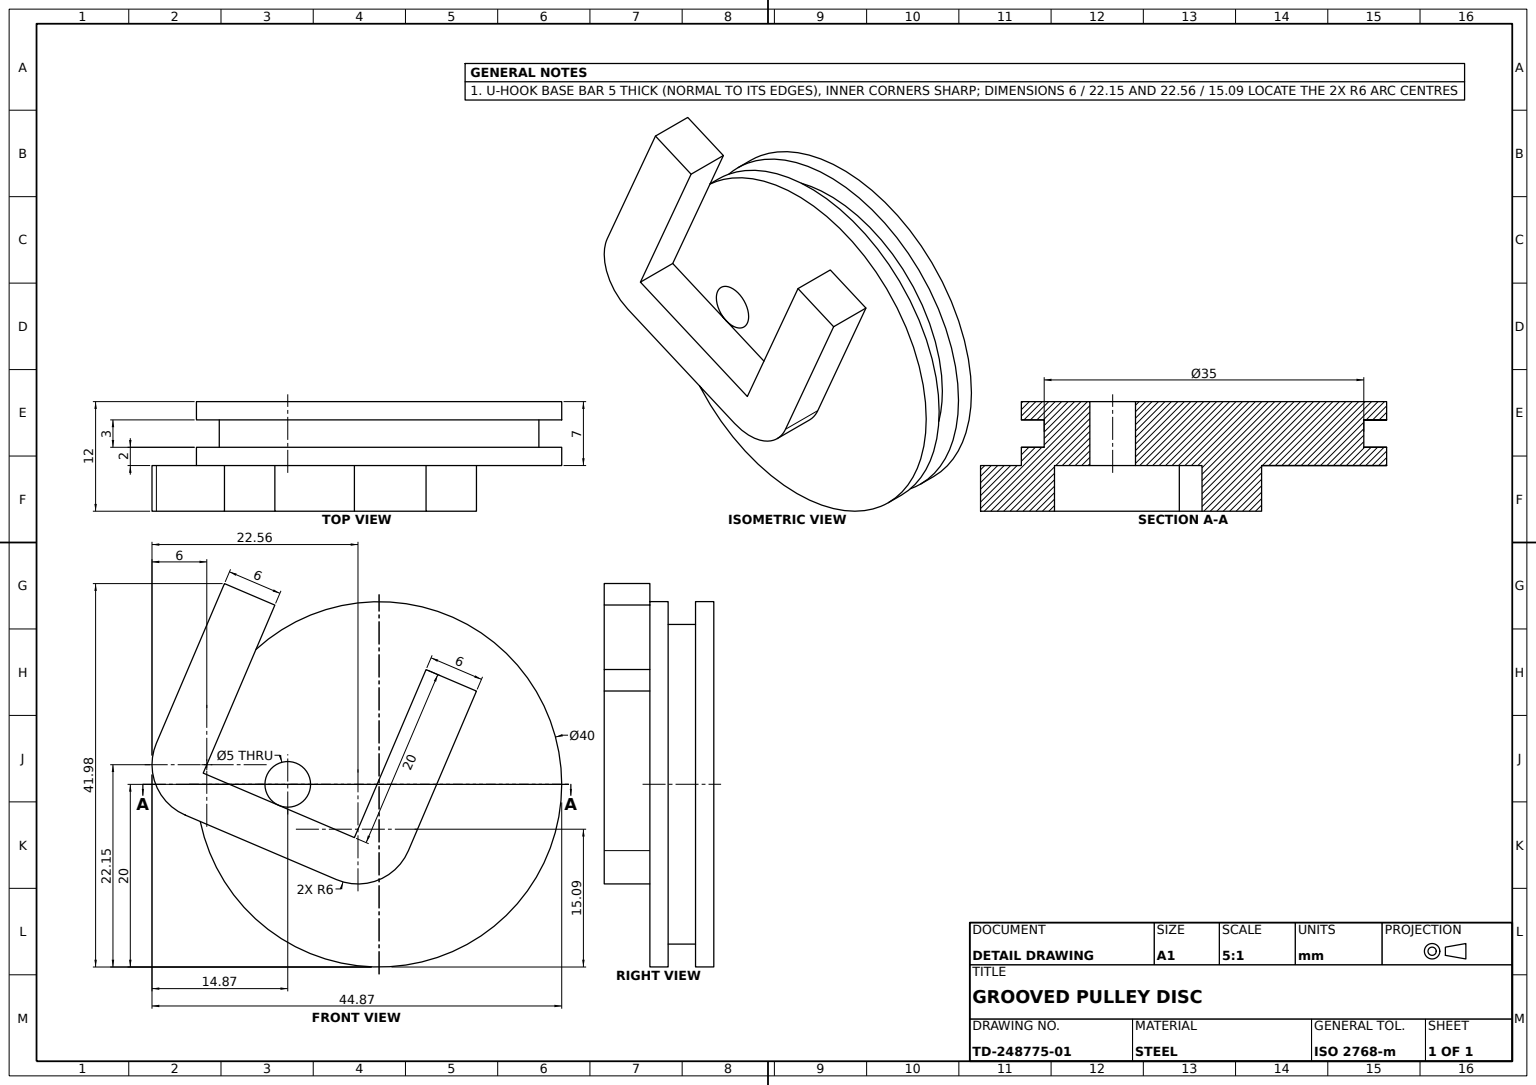
SolidWorks part; units mm, degrees
material "Plain Carbon Steel"
ref_plane "Front Plane" through (0, 0, 0) normal (0, 0, 1) x (1, 0, 0)
ref_plane "Top Plane" through (0, 0, 0) normal (0, 1, 0) x (1, 0, 0)
ref_plane "Right Plane" through (0, 0, 0) normal (1, 0, 0) x (0, 0, -1)
sketch "Disc Profile Ø40" plane through (0, 0, 0) normal (0, 0, 1) x (1, 0, 0)
  circle A0 centre (0, 0) radius 20
  dimension "D1" = 40
extrude "Disc Ø40x7" add sketch "Disc Profile Ø40" along normal mid plane 7
sketch "Rim Groove Profile" plane through (0, 0, 0) normal (1, 0, 0) x (0, 0, -1)
  line L0 (3.5, 20) -> (-3.5, 20) construction
  line L1 (-1.5, 20) -> (1.5, 20)
  line L2 (-1.5, 20) -> (-1.5, 17.5)
  line L3 (-1.5, 17.5) -> (1.5, 17.5)
  line L4 (1.5, 20) -> (1.5, 17.5)
  line L5 (-3.5, 20) -> (-3.5, -20) construction
  line L6 (3.5, -20) -> (3.5, 20) construction
  line L7 (-14.7566, 0) -> (34.8551, 0)
  dimension "D1" = 2.5
  dimension "D2" = 2
  dimension "D3" = 2
  dimension "D4" = 36.3551
  dimension "D5" = 13.2566
revolve "Rim Groove" cut sketch "Rim Groove Profile" angle 360 about L7
sketch "Through Hole Profile" plane through (0, 0, 3.5) normal (0, 0, 1) x (1, 0, 0)
  circle A0 centre (-10, 0) radius 2.5
  circle A1 centre (0, 0) radius 20 construction
  dimension "D2" = 5
  dimension "D1" = 10
  dimension "D3" = 10
extrude "Through Hole" cut sketch "Through Hole Profile" against normal blind 47
sketch "U Hook Profile" plane through (0, 0, 3.5) normal (0, 0, 1) x (1, 0, 0)
  line L0 (-19.2592, 1.2315) -> (-2.7025, -5.8306)
  line L1 (-2.7025, -5.8306) -> (5.1443, 12.5658)
  line L2 (-24.3858, 4.5054) -> (-16.9313, 21.982)
  line L3 (-19.2592, 1.2315) -> (-11.4124, 19.6279)
  line L6 (3.2088, -7.2648) -> (10.6633, 10.2117)
  line L7 (-16.9313, 21.982) -> (-11.4124, 19.6279)
  line L8 (5.1443, 12.5658) -> (10.6633, 10.2117)
  line L9 (-21.2209, -3.3676) -> (-4.6642, -10.4297)
  circle A0 centre (-10, 0) radius 2.5
  arc A1 (-4.6642, -10.4297) -> (3.2088, -7.2648) centre (-2.3101, -4.9108) ccw
  arc A2 (-21.2209, -3.3676) -> (-24.3858, 4.5054) centre (-18.8669, 2.1513) cw
  circle A3 centre (-10, 0) radius 2.5 construction
  point P9 (0, 0)
  dimension "D1" = 5
  dimension "D8" = 6
  dimension "D2" = 5
  dimension "D3" = 25
  dimension "D4" = 30
  dimension "D5" = 18
  dimension "D6" = 9
  dimension "D7" = 15
  dimension "D9" = 5.3358
  dimension "D10" = 7.2975
  dimension "D11" = 20.6633
extrude "U Hook Boss" add sketch "U Hook Profile" along normal blind 5 contours L9 A1 L6 L8 L1 L0 L3 L7 L2 A2
